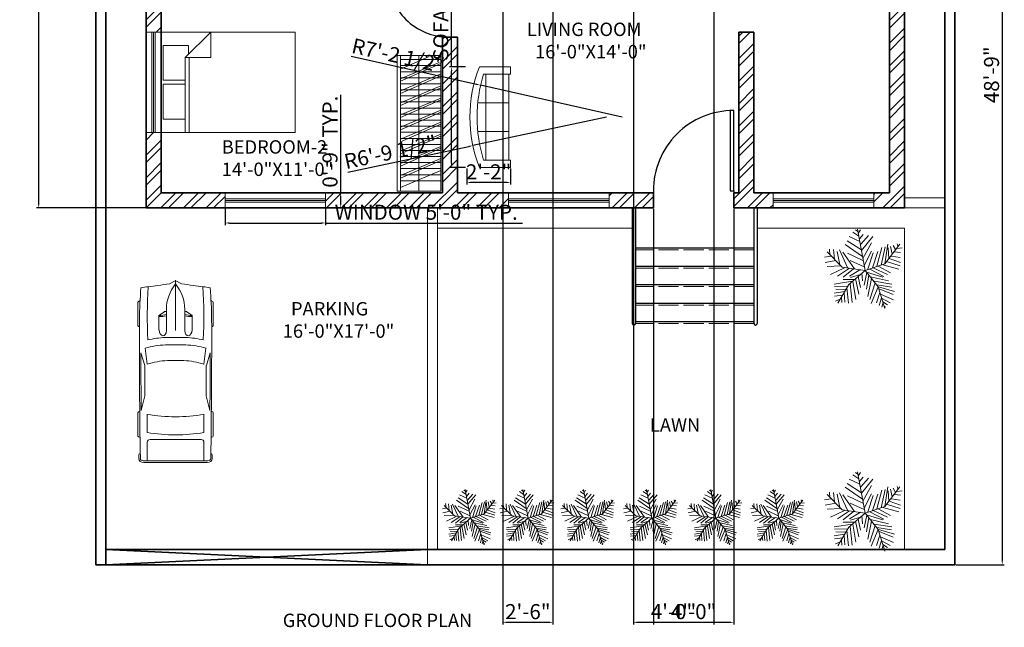
# Model space of a CAD drawing. Units: inches. Extents: x 451 to 1761, y 2292 to 3014.
# Tile 1 of 3: x 451 to 1039, y 2292 to 2655. Entities that reach past the tile are written whole.
import ezdxf

# ---------------------------------------------------------------- set-up
doc = ezdxf.new("R2010")
doc.units = ezdxf.units.IN
doc.linetypes.add('ACAD_ISO02W100', pattern=[15, 12, -3])
for name, color, linetype, lineweight in [('A-ANNO-DIMS', 2, 'Continuous', 18), ('A-ANNO-TEXT', 7, 'Continuous', 25), ('A-AREA-IDEN', 7, 'Continuous', 18), ('A-DOOR', 4, 'Continuous', 25), ('A-FLOR-CASE', 9, 'Continuous', 18), ('A-FLOR-CASE-PATT', 252, 'Continuous', 13), ('A-FLOR-STRS', 7, 'Continuous', 25), ('A-FLOR-STRS-HIDN', 8, 'ACAD_ISO02W100', 13), ('A-FURN', 8, 'Continuous', 18), ('A-GLAZ', 244, 'Continuous', 18), ('A-WALL', 7, 'Continuous', 35), ('A-WALL-PATT', 252, 'Continuous', 13), ('C-PROP', 7, 'Continuous', 35), ('C-SITE', 8, 'Continuous', 18), ('C-SITE-VEHC', 9, 'Continuous', 18), ('L-PLNT', 3, 'Continuous', 18)]:
    doc.layers.add(name, color=color, linetype=linetype, lineweight=lineweight)
doc.styles.get("Standard").update_dxf_attribs({"font": 'arial.ttf'})
doc.dimstyles.new('ISO-25', dxfattribs={"dimtxt": 9, "dimasz": 2.5, "dimexe": 1.25, "dimexo": 0.625, "dimtad": 1, "dimlunit": 3, "dimtxsty": 'Standard', "dimcen": 2.5, "dimadec": 0, "dimazin": 0, "dimtfac": 1, "dimtmove": 0, "dimatfit": 3, "dimfxl": 1, "dimarcsym": 0})

# ---------------------------------------------------------------- blocks, each defined once
blk = doc.blocks.new('*U3')
for p, q in [((0, 0), (0, 6)), ((40, 0), (40, 6))]:
    blk.add_line(p, q)
blk.add_lwpolyline([(0, 0), (0, -40), (1.75, -40), (1.75, 0)], close=True)
blk.add_arc((0, 0), 40, 270, 0)
blk = doc.blocks.new('Bed - Queen')
for p, q in [((0, -80.00003), (0, 0)), ((0, 0), (59.99999, 0)), ((59.99999, 0), (59.99999, -80.00003)), ((7.99999, -1.2), (28.79998, -1.2)), ((7.99999, -14.4), (7.99999, -1.2)), ((28.79998, -1.2), (28.79998, -14.4)), ((31.19999, -1.2), (51.99999, -1.2)), ((31.19999, -14.4), (31.19999, -1.2)), ((51.99999, -1.2), (51.99999, -16.4)), ((0, -14.4), (44.8, -14.4)), ((44.8, -16.8), (0, -16.8)), ((59.99999, -29.6), (44.8, -14.4)), ((44.8, -14.4), (44.8, -29.6)), ((51.99999, -16.4), (46.79936, -16.4)), ((44.8, -29.6), (59.99999, -29.6)), ((59.99999, -80.00003), (0, -80.00003))]:
    blk.add_line(p, q)
blk = doc.blocks.new('Sofa - Roundback 7 ft.')
for p, q in [((-12.00002, -32.4421), (-12.00003, -6.5971)), ((11.99997, -32.4421), (11.99998, -6.5971)), ((-36.000027, -34), (-36.000027, -11.4696)), ((-35.999844, -13.3819), (35.9998, -13.3819)), ((35.99998, -34), (35.99998, -11.4696)), ((-36.000027, -32.4421), (35.99998, -32.4421))]:
    blk.add_line(p, q)
for points in [[(-36.000027, -34), (-42.000027, -34), (-42.000027, -8)], [(41.99998, -8), (41.99998, -34), (35.99998, -34)]]:
    blk.add_lwpolyline(points)
for centre, radius, start, end in [((0, -114.25), 114.25, 68.43141, 111.5686), ((-0.00001, -127.1968), 121.1968, 72.72033, 107.2797)]:
    blk.add_arc(centre, radius, start, end)
blk = doc.blocks.new('*U12')
for p, q in [((-10.186, 53.64), (-13.084, 55.962)), ((0, 0), (-10.5, 57)), ((-9.099, 51.782), (-6.563, 55.962)), ((-7.288, 39.707), (-21.778, 46.673)), ((-8.737, 47.138), (-17.069, 52.711)), ((-7.65, 43.423), (-2.578, 49.46)), ((-5.839, 35.992), (4.667, 48.067)), ((-5.114, 27.632), (10.463, 46.673)), ((-48.585, 21.131), (-49.309, 29.026)), ((-43.513, 28.561), (-42.427, 15.558)), ((-35.544, 28.097), (-24.314, 3.947)), ((-3.665, 19.273), (-27.574, 35.527)), ((-5.114, 28.097), (-24.676, 40.636)), ((-2.941, 16.486), (8.652, 37.85)), ((16.259, 5.805), (23.142, 31.348)), ((22.055, 7.198), (27.489, 32.277)), ((27, 9), (48, 36)), ((27.127, 9.056), (31.112, 35.992)), ((31.836, 30.883), (32.561, 16.486)), ((35.096, 32.741), (37.27, 22.524)), ((38.719, 34.134), (41.979, 28.561)), ((43.791, 29.954), (51.036, 30.883)), ((44.153, 36.456), (45.239, 32.741)), ((-47.498, 19.737), (-55.83, 18.344)), ((-40.615, 13.7), (-55.105, 10.913)), ((-31.5, 4.5), (-52.5, 25.5)), ((-38.442, 26.239), (-34.819, 7.663)), ((-14.533, 2.09), (-30.834, 25.31)), ((-24.314, 23.917), (-2.941, 13.7)), ((-20.691, 13.7), (-1.129, 4.876)), ((-1.129, 6.734), (9.014, 26.704)), ((3.942, 1.625), (11.187, 24.381)), ((10.101, 3.483), (17.708, 26.239)), ((33.285, 16.486), (48.862, 10.913)), ((36.183, 19.737), (48.137, 17.88)), ((40.53, 25.775), (48.862, 24.846)), ((-33.37, 6.269), (-52.207, 5.34)), ((-28.299, 3.483), (-47.86, -5.805)), ((-21.416, 3.018), (-38.079, -8.128)), ((0, 0), (-31.5, 4.5)), ((-15.982, 2.09), (-30.11, -9.521)), ((0, 0), (-22.5, -19.5)), ((-6.563, 1.161), (-21.416, -8.128)), ((0, 0), (27, 9)), ((0, 0), (18, -22.5)), ((6.478, 1.625), (26.04, -8.592)), ((11.187, 3.483), (30.749, -5.805)), ((18.07, 5.805), (35.096, -3.483)), ((24.229, 7.663), (46.688, 1.625)), ((29.662, 12.307), (48.137, 6.269)), ((-15.257, -12.772), (-30.11, -12.772)), ((-6.563, -5.805), (-19.967, -9.985)), ((-13.446, -11.378), (-8.737, -32.741)), ((-9.461, -8.592), (-6.201, -23.453)), ((-4.752, -3.483), (-3.665, -14.629)), ((2.493, -3.019), (-1.491, -20.202)), ((1.769, -2.555), (24.229, -9.521)), ((5.029, -6.27), (2.131, -25.775)), ((9.014, -11.378), (3.58, -35.992)), ((7.565, -9.056), (32.198, -14.629)), ((-17.431, -15.094), (-42.789, -18.809)), ((-24.314, -21.596), (-42.427, -22.06)), ((-26.849, -26.24), (-40.253, -25.775)), ((-22.5, -19.5), (-37.5, -45)), ((-25.038, -23.918), (-22.865, -45.281)), ((-20.691, -18.345), (-17.793, -44.352)), ((-17.069, -15.094), (-12.721, -40.172)), ((14.085, -16.951), (6.478, -40.172)), ((18.07, -22.524), (8.289, -45.745)), ((12.274, -15.094), (36.907, -18.809)), ((16.259, -19.738), (36.183, -22.989)), ((18, -22.5), (27, -52.5)), ((18.433, -22.524), (40.53, -29.026)), ((19.157, -25.311), (38.719, -33.206)), ((-28.299, -29.026), (-42.789, -31.348)), ((-30.834, -34.135), (-42.427, -35.528)), ((-34.457, -39.708), (-40.978, -42.494)), ((-32.646, -36.921), (-31.921, -44.352)), ((-29.023, -30.884), (-27.936, -43.887)), ((20.244, -30.419), (15.897, -44.816)), ((22.78, -37.85), (19.519, -48.532)), ((21.331, -32.741), (39.081, -40.636)), ((22.78, -38.314), (34.372, -44.816)), ((24.591, -45.745), (23.142, -50.854)), ((24.591, -43.423), (30.749, -47.603)), ((26.764, -49.925), (28.213, -50.854))]:
    blk.add_line(p, q)
blk = doc.blocks.new('*D13')
at = {"layer": 'A-ANNO-DIMS', "color": 0, "lineweight": -2, "transparency": 16777216}
for p, q in [((1010.42, 2914.76), (1039.33, 2914.76)), ((1038.08, 2912.26), (1038.08, 2332.26)), ((1010.42, 2329.76), (1039.33, 2329.76))]:
    blk.add_line(p, q, dxfattribs=at)
at = {"layer": 'A-ANNO-DIMS', "color": 0, "transparency": 16777216}
for points in [[(1037.66, 2912.26), (1038.49, 2912.26), (1038.08, 2914.76)], [(1037.66, 2332.26), (1038.49, 2332.26), (1038.08, 2329.76)]]:
    blk.add_solid(points, dxfattribs=at)
at = {"layer": 'Defpoints', "color": 0, "transparency": 16777216}
for p in [(1009.79, 2914.76), (1009.79, 2329.76), (1038.08, 2329.76)]:
    blk.add_point(p, dxfattribs=at)
at = {"layer": 'A-ANNO-DIMS', "color": 0, "transparency": 16777216, "insert": (1032.86, 2622.26), "char_height": 9, "attachment_point": 5, "rotation": 90}
blk.add_mtext('48\'-9"', dxfattribs=at)
blk = doc.blocks.new('*U18')
for p, q in [((21.1, 37.4), (21.1, 36.8)), ((46.6, 38.9), (22.4, 38.9)), ((47.8, 37.4), (47.8, 37.4)), ((70, 31.5), (86.4, 29.4)), ((88, 31.9), (74.8, 35.9)), ((134.3, 35.6), (119.3, 31.8)), ((135.5, 37.1), (135.5, 37.4)), ((136.7, 38.9), (160.9, 38.9)), ((162.1, 37.4), (162.1, 36.8)), ((186.5, -33.5), (186.5, 33.5)), ((188.4, -32.8), (188.4, 32.8)), ((138.4, 29.4), (157.2, 29.4)), ((164.5, 26.4), (164.5, -26.4)), ((186.5, 29.4), (167, 29.4)), ((32.1, 9.5), (32.1, 11.2)), ((32.3, 11.6), (36.1, 17.2)), ((36.1, 17.2), (50.9, 17.2)), ((58.9, -10.8), (58.9, 10.8)), ((66.6, -10.5), (66.6, 10.5)), ((186.5, -10.5), (186.5, 10.5)), ((3.3, 6.1), (0.1, 0.4)), ((29.8, 9.5), (51.7, 9.5)), ((82.7, 8.5), (82.7, -8.5)), ((0, 0), (51.7, 0)), ((0.1, -0.4), (3.3, -6.1)), ((29.8, -9.5), (51.7, -9.5)), ((32.1, -9.5), (32.1, -11.2)), ((32.3, -11.6), (36.1, -17.2)), ((36.1, -17.2), (50.9, -17.2)), ((86.4, -29.4), (70, -31.5)), ((157.2, -29.4), (138.4, -29.4)), ((167, -29.4), (186.5, -29.4)), ((21.1, -37.4), (21.1, -36.8)), ((46.6, -38.9), (22.4, -38.9)), ((47.8, -37.4), (47.8, -37.4)), ((88, -31.9), (74.8, -35.9)), ((134.3, -35.6), (119.3, -31.8)), ((135.5, -37.1), (135.5, -37.4)), ((136.7, -38.9), (160.9, -38.9)), ((162.1, -37.4), (162.1, -36.8))]:
    blk.add_line(p, q)
for centre, major_axis, ratio, start_param, end_param in [((266, -27.5), (0, 313.3), 0.842304, 1.367076, 1.39176), ((41.2, -490.9), (0, 528.2), 0.842304, 0.00281, 0.075598), ((22.4, 37.4), (0, -1.48), 0.842304, 3.141593, 4.712389), ((64.5, -10555.6), (0, 10593), 0.842304, -0.013397, 0.002797), ((46.6, 37.4), (0, 1.48), 0.842304, -1.570796, 0), ((135.3, 5.4), (0, 81.8), 0.842304, 1.245306, 1.50788), ((64.5, -10555.6), (0, -10591.5), 0.842304, 3.133765, 3.140441), ((95.8, -3666.4), (0, -3698.2), 0.842304, 3.134049, 3.144098), ((136.7, 37.4), (0, -1.48), 0.842304, 3.141593, 4.712389), ((160.9, 37.4), (0, 1.48), 0.842304, -1.570796, 0), ((180.6, 35.8), (0, 2.22), 0.842304, -0.013017, 1.249894), ((64.5, -10556.4), (0, 10595.3), 0.842304, -0.013397, -0.013017), ((184, 32.8), (0, -5.25), 0.842304, 1.570796, 3.128196), ((184, 33.5), (0, -2.96), 0.842304, 1.570796, 3.128196), ((259.2, -27.5), (0, -305.3), 0.842304, 4.528606, 4.561838), ((37.5, -594), (0, -623.3), 0.842304, 3.096046, 3.200911), ((134.4, 5.4), (0, -89.8), 0.842304, 4.449482, 4.652344), ((149.6, 2.8), (0, -79.6), 0.842304, 4.372215, 4.640744), ((17.1, 0), (0, 147), 0.842304, 4.511394, 4.913384), ((35.9, 0), (0, 147), 0.842304, 4.511394, 4.913384), ((167, 26.4), (0, 2.96), 0.842304, 0, 1.570796), ((-204.5, 52.4), (0, -251), 0.842304, 1.385369, 1.434372), ((32.7, 11.2), (0, 0.74), 0.842304, 0.879714, 1.570796), ((13, 17), (0, 27.4), 0.842304, 4.435146, 4.718221), ((14.2, 17), (0, 27.4), 0.842304, 4.435146, 4.718221), ((50.8, 13.3), (6.34, -0.36), 0.603834, -1.395552, 1.581315), ((0.6, 0), (0, -0.74), 0.842304, 4.131459, 5.293319), ((29.8, -46.7), (0, 56.2), 0.842304, 0, 0.590319), ((-204.5, -52.4), (0, 251), 0.842304, -1.434372, -1.385369), ((29.8, 46.7), (0, 56.2), 0.842304, 2.551274, 3.141593), ((13, -17), (0, -27.4), 0.842304, 1.564964, 1.848039), ((14.2, -17), (0, -27.4), 0.842304, 1.564964, 1.848039), ((149.6, -2.8), (0, -79.6), 0.842304, -1.499151, -1.230623), ((259.2, 27.5), (0, 305.3), 0.842304, 1.721348, 1.754579), ((32.7, -11.2), (0, -0.74), 0.842304, 4.712389, 5.403472), ((134.4, -5.4), (0, -89.8), 0.842304, -1.510751, -1.307889), ((135.3, -5.4), (0, -81.8), 0.842304, -1.50788, -1.245306), ((266, 27.5), (0, 313.3), 0.842304, 1.749832, 1.774517), ((37.5, 594), (0, -623.3), 0.842304, -0.059319, 0.045547), ((167, -26.4), (0, -2.96), 0.842304, 4.712389, 6.283185), ((41.2, 490.9), (0, -528.2), 0.842304, -0.075598, -0.00281), ((22.4, -37.4), (0, 1.48), 0.842304, 1.570796, 3.141593), ((64.5, 10555.6), (0, 10593), 0.842304, 3.138796, 3.15499), ((46.6, -37.4), (0, -1.48), 0.842304, 0, 1.570796), ((64.5, 10555.6), (0, -10591.5), 0.842304, 0.001152, 0.007828), ((95.8, 3666.4), (0, -3698.2), 0.842304, -0.002505, 0.007544), ((136.7, -37.4), (0, -1.48), 0.842304, -1.570796, 0), ((160.9, -37.4), (0, 1.48), 0.842304, 3.141593, 4.712389), ((180.6, -35.8), (0, -2.22), 0.842304, -1.249894, 0.013017), ((64.5, 10556.4), (0, 10595.3), 0.842304, 3.15461, 3.15499), ((184, -32.8), (0, -5.25), 0.842304, 0.013397, 1.570796), ((184, -33.5), (0, 2.96), 0.842304, 3.15499, 4.712389)]:
    blk.add_ellipse(centre, major_axis=major_axis, ratio=ratio, start_param=start_param, end_param=end_param)
at = {"extrusion": (0, 0, -1)}
blk.add_ellipse((50.8, -13.3), major_axis=(6.34, 0.36), ratio=0.603834, start_param=-1.395552, end_param=1.581315, dxfattribs=at)
blk = doc.blocks.new('WIN-60IN')
for p, q in [((0, 5.5), (60, 5.5)), ((0, 4.5), (60, 4.5)), ((0, 3.5), (60, 3.5))]:
    blk.add_line(p, q)
blk.add_lwpolyline([(0, 0), (0, 9), (60, 9), (60, 0)], close=True)
blk = doc.blocks.new('*D24')
at = {"layer": 'A-ANNO-DIMS', "color": 0, "lineweight": -2, "transparency": 16777216}
for p, q in [((574.03, 2542.13), (574.03, 2532.51)), ((634.03, 2542.13), (634.03, 2532.51)), ((576.53, 2533.76), (631.53, 2533.76)), ((634.03, 2533.76), (751.66, 2533.76))]:
    blk.add_line(p, q, dxfattribs=at)
at = {"layer": 'A-ANNO-DIMS', "color": 0, "transparency": 16777216}
for points in [[(576.53, 2534.18), (576.53, 2533.34), (574.03, 2533.76)], [(631.53, 2534.18), (631.53, 2533.34), (634.03, 2533.76)]]:
    blk.add_solid(points, dxfattribs=at)
at = {"layer": 'Defpoints', "color": 0, "transparency": 16777216}
for p in [(574.03, 2542.76), (634.03, 2542.76), (634.03, 2533.76)]:
    blk.add_point(p, dxfattribs=at)
at = {"layer": 'A-ANNO-DIMS', "color": 0, "transparency": 16777216, "insert": (694.1, 2539.04), "char_height": 9, "attachment_point": 5}
blk.add_mtext('WINDOW 5\'-0" TYP.', dxfattribs=at)
blk = doc.blocks.new('*D25')
at = {"layer": 'A-ANNO-DIMS', "color": 0, "lineweight": -2, "transparency": 16777216}
for p, q in [((643.03, 2551.76), (643.03, 2610.37)), ((634.65, 2551.76), (644.28, 2551.76)), ((643.03, 2545.26), (643.03, 2549.26)), ((634.65, 2542.76), (644.28, 2542.76))]:
    blk.add_line(p, q, dxfattribs=at)
at = {"layer": 'A-ANNO-DIMS', "color": 0, "transparency": 16777216}
for points in [[(642.61, 2549.26), (643.44, 2549.26), (643.03, 2551.76)], [(642.61, 2545.26), (643.44, 2545.26), (643.03, 2542.76)]]:
    blk.add_solid(points, dxfattribs=at)
at = {"layer": 'Defpoints', "color": 0, "transparency": 16777216}
for p in [(634.03, 2551.76), (643.03, 2551.76), (634.03, 2542.76)]:
    blk.add_point(p, dxfattribs=at)
at = {"layer": 'A-ANNO-DIMS', "color": 0, "transparency": 16777216, "insert": (637.81, 2582.31), "char_height": 9, "attachment_point": 5, "rotation": 90}
blk.add_mtext('0\'-9" TYP.', dxfattribs=at)
blk = doc.blocks.new('*D32')
at = {"layer": 'A-ANNO-DIMS', "color": 0, "lineweight": -2, "transparency": 16777216}
for p, q in [((709.28, 2626.98), (709.28, 2692.34)), ((717.66, 2626.98), (708.03, 2626.98)), ((709.28, 2569.48), (709.28, 2624.48)), ((717.66, 2566.98), (708.03, 2566.98))]:
    blk.add_line(p, q, dxfattribs=at)
at = {"layer": 'A-ANNO-DIMS', "color": 0, "transparency": 16777216}
for points in [[(708.87, 2624.48), (709.7, 2624.48), (709.28, 2626.98)], [(708.87, 2569.48), (709.7, 2569.48), (709.28, 2566.98)]]:
    blk.add_solid(points, dxfattribs=at)
at = {"layer": 'Defpoints', "color": 0, "transparency": 16777216}
for p in [(709.28, 2626.98), (718.28, 2626.98), (718.28, 2566.98)]:
    blk.add_point(p, dxfattribs=at)
at = {"layer": 'A-ANNO-DIMS', "color": 0, "transparency": 16777216, "insert": (704, 2660.91), "char_height": 9, "attachment_point": 5, "rotation": 90}
blk.add_mtext('SOFA 5\'-0"', dxfattribs=at)
blk = doc.blocks.new('*D33')
at = {"layer": 'A-ANNO-DIMS', "color": 0, "lineweight": -2, "transparency": 16777216}
for p, q in [((718.28, 2566.36), (718.28, 2556.73)), ((744.47, 2566.36), (744.47, 2556.73)), ((741.97, 2557.98), (720.78, 2557.98))]:
    blk.add_line(p, q, dxfattribs=at)
at = {"layer": 'A-ANNO-DIMS', "color": 0, "transparency": 16777216}
for points in [[(720.78, 2558.4), (720.78, 2557.57), (718.28, 2557.98)], [(741.97, 2558.4), (741.97, 2557.57), (744.47, 2557.98)]]:
    blk.add_solid(points, dxfattribs=at)
at = {"layer": 'Defpoints', "color": 0, "transparency": 16777216}
for p in [(718.28, 2566.98), (744.47, 2566.98), (718.28, 2557.98)]:
    blk.add_point(p, dxfattribs=at)
at = {"layer": 'A-ANNO-DIMS', "color": 0, "transparency": 16777216, "insert": (731.38, 2563.13), "char_height": 9, "attachment_point": 5}
blk.add_mtext('2\'-2"', dxfattribs=at)
blk = doc.blocks.new('*D35')
at = {"layer": 'A-ANNO-DIMS', "color": 0, "lineweight": -2, "transparency": 16777216}
for p, q in [((526.17, 2914.76), (461.44, 2914.76)), ((462.69, 2545.26), (462.69, 2912.26)), ((526.17, 2542.76), (461.44, 2542.76))]:
    blk.add_line(p, q, dxfattribs=at)
at = {"layer": 'A-ANNO-DIMS', "color": 0, "transparency": 16777216}
for points in [[(462.27, 2912.26), (463.11, 2912.26), (462.69, 2914.76)], [(462.27, 2545.26), (463.11, 2545.26), (462.69, 2542.76)]]:
    blk.add_solid(points, dxfattribs=at)
at = {"layer": 'Defpoints', "color": 0, "transparency": 16777216}
for p in [(462.69, 2914.76), (526.79, 2914.76), (526.79, 2542.76)]:
    blk.add_point(p, dxfattribs=at)
at = {"layer": 'A-ANNO-DIMS', "color": 0, "transparency": 16777216, "insert": (457.47, 2728.76), "char_height": 9, "attachment_point": 5, "rotation": 90}
blk.add_mtext('31\'-0"', dxfattribs=at)
blk = doc.blocks.new('*D37')
at = {"layer": 'A-ANNO-DIMS', "color": 0, "lineweight": -2, "transparency": 16777216}
for p, q in [((829.79, 2542.13), (829.79, 2294.1)), ((877.79, 2542.13), (877.79, 2294.1)), ((832.29, 2295.35), (875.29, 2295.35))]:
    blk.add_line(p, q, dxfattribs=at)
at = {"layer": 'A-ANNO-DIMS', "color": 0, "transparency": 16777216}
for points in [[(832.29, 2295.77), (832.29, 2294.93), (829.79, 2295.35)], [(875.29, 2295.77), (875.29, 2294.93), (877.79, 2295.35)]]:
    blk.add_solid(points, dxfattribs=at)
at = {"layer": 'Defpoints', "color": 0, "transparency": 16777216}
for p in [(829.79, 2542.76), (877.79, 2542.76), (877.79, 2295.35)]:
    blk.add_point(p, dxfattribs=at)
at = {"layer": 'A-ANNO-DIMS', "color": 0, "transparency": 16777216, "insert": (853.79, 2300.57), "char_height": 9, "attachment_point": 5}
blk.add_mtext('4\'-0"', dxfattribs=at)
blk = doc.blocks.new('*D38')
at = {"layer": 'A-ANNO-DIMS', "color": 0, "lineweight": -2, "transparency": 16777216}
for p, q in [((817.79, 2776.13), (817.79, 2294.1)), ((865.79, 2776.13), (865.79, 2294.1)), ((820.29, 2295.35), (863.29, 2295.35))]:
    blk.add_line(p, q, dxfattribs=at)
at = {"layer": 'A-ANNO-DIMS', "color": 0, "transparency": 16777216}
for points in [[(820.29, 2295.77), (820.29, 2294.93), (817.79, 2295.35)], [(863.29, 2295.77), (863.29, 2294.93), (865.79, 2295.35)]]:
    blk.add_solid(points, dxfattribs=at)
at = {"layer": 'Defpoints', "color": 0, "transparency": 16777216}
for p in [(817.79, 2776.76), (865.79, 2776.76), (865.79, 2295.35)]:
    blk.add_point(p, dxfattribs=at)
at = {"layer": 'A-ANNO-DIMS', "color": 0, "transparency": 16777216, "insert": (841.79, 2300.57), "char_height": 9, "attachment_point": 5}
blk.add_mtext('4\'-0"', dxfattribs=at)
blk = doc.blocks.new('*D39')
at = {"layer": 'A-ANNO-DIMS', "color": 0, "lineweight": -2, "transparency": 16777216}
for p, q in [((739.79, 2812.13), (739.79, 2294.1)), ((769.79, 2812.13), (769.79, 2294.1)), ((742.29, 2295.35), (767.29, 2295.35))]:
    blk.add_line(p, q, dxfattribs=at)
at = {"layer": 'A-ANNO-DIMS', "color": 0, "transparency": 16777216}
for points in [[(742.29, 2295.77), (742.29, 2294.93), (739.79, 2295.35)], [(767.29, 2295.77), (767.29, 2294.93), (769.79, 2295.35)]]:
    blk.add_solid(points, dxfattribs=at)
at = {"layer": 'Defpoints', "color": 0, "transparency": 16777216}
for p in [(739.79, 2812.76), (769.79, 2812.76), (769.79, 2295.35)]:
    blk.add_point(p, dxfattribs=at)
at = {"layer": 'A-ANNO-DIMS', "color": 0, "transparency": 16777216, "insert": (754.79, 2300.57), "char_height": 9, "attachment_point": 5}
blk.add_mtext('2\'-6"', dxfattribs=at)
blk = doc.blocks.new('*D48')
at = {"layer": 'A-ANNO-DIMS', "color": 0, "lineweight": -2, "transparency": 16777216}
for p, q in [((649.21, 2633.44), (724.15, 2616.56)), ((811.04, 2596.98), (726.59, 2616.01))]:
    blk.add_line(p, q, dxfattribs=at)
at = {"layer": 'A-ANNO-DIMS', "color": 0, "transparency": 16777216}
blk.add_solid([(724.24, 2616.96), (724.06, 2616.15), (726.59, 2616.01)], dxfattribs=at)
at = {"layer": 'Defpoints', "color": 0, "transparency": 16777216}
for p in [(726.59, 2616.01), (811.04, 2596.98)]:
    blk.add_point(p, dxfattribs=at)
at = {"layer": 'A-ANNO-DIMS', "color": 0, "transparency": 16777216, "insert": (677.08, 2632.57), "char_height": 9, "attachment_point": 5, "rotation": 347.30544}
blk.add_mtext('R7\'-2 1/2"', dxfattribs=at)
blk = doc.blocks.new('*D49')
at = {"layer": 'A-ANNO-DIMS', "color": 0, "lineweight": -2, "transparency": 16777216}
for p, q in [((801.8, 2596.98), (721.98, 2580)), ((647.3, 2564.11), (719.53, 2579.48))]:
    blk.add_line(p, q, dxfattribs=at)
at = {"layer": 'A-ANNO-DIMS', "color": 0, "transparency": 16777216}
blk.add_solid([(719.44, 2579.89), (719.62, 2579.07), (721.98, 2580)], dxfattribs=at)
at = {"layer": 'Defpoints', "color": 0, "transparency": 16777216}
for p in [(801.8, 2596.98), (721.98, 2580)]:
    blk.add_point(p, dxfattribs=at)
at = {"layer": 'A-ANNO-DIMS', "color": 0, "transparency": 16777216, "insert": (672.98, 2574.97), "char_height": 9, "attachment_point": 5, "rotation": 12.01201}
blk.add_mtext('R6\'-9 1/2"', dxfattribs=at)

msp = doc.modelspace()

# ---------------------------------------------------------------- hatches: boundary and pattern name
at = {"layer": 'A-FLOR-CASE-PATT'}
h = msp.add_hatch(dxfattribs=at)
h.set_pattern_fill('ANSI31', color=256, scale=2.09659, angle=-22.1278, style=0)
h.paths.add_polyline_path([(678.791, 2552.759), (702.791, 2562.883), (702.791, 2627.905), (699.385, 2633.693), (678.791, 2625.006)])
h = msp.add_hatch(dxfattribs=at)
h.set_pattern_fill('ANSI31', color=256, scale=2.08217, angle=-21.2114, style=0)
h.paths.add_polyline_path([(678.791, 2556.222), (702.791, 2566.801), (702.791, 2631.824), (690.643, 2633.693), (678.791, 2628.469)])
h = msp.add_hatch(dxfattribs=at)
h.set_pattern_fill('ANSI31', color=256, scale=1.13999, angle=-45, style=0)
h.paths.add_polyline_path([(678.791, 2556.222), (702.791, 2556.222), (702.791, 2632.23), (678.791, 2632.23)])
at = {"layer": 'A-WALL-PATT'}
h = msp.add_hatch(dxfattribs=at)
h.set_pattern_fill('ANSI32', color=256)
h.paths.add_polyline_path([(703.791, 2551.759), (634.026, 2551.759), (634.026, 2542.759), (743.266, 2542.759), (743.266, 2551.759), (712.791, 2551.759), (712.791, 2644.759), (707.391, 2644.759), (703.791, 2644.759)])
h.paths.add_polyline_path([(535.791, 2551.759), (535.791, 2587.758), (526.791, 2587.758), (526.791, 2542.759), (574.026, 2542.759), (574.026, 2551.759)])
h.paths.add_polyline_path([(526.791, 2647.758), (535.791, 2647.758), (535.791, 2683.759), (619.791, 2683.759), (619.791, 2692.759), (535.791, 2692.759), (535.791, 2726.772), (526.791, 2726.772)])
h.paths.add_polyline_path([(649.791, 2692.759), (649.791, 2683.759), (703.791, 2683.759), (703.791, 2680.759), (712.791, 2680.759), (712.791, 2752.759), (712.791, 2764.759), (703.791, 2764.759), (703.791, 2761.759), (535.791, 2761.759), (535.791, 2804.959), (526.791, 2804.959), (526.791, 2747.772), (535.791, 2747.772), (535.791, 2752.759), (703.791, 2752.759), (703.791, 2692.759)])
h.paths.add_polyline_path([(781.791, 2785.759), (781.791, 2905.759), (811.791, 2905.759), (811.791, 2914.759), (763.791, 2914.759), (763.791, 2905.759), (772.791, 2905.759), (772.791, 2821.759), (769.791, 2821.759), (769.791, 2812.759), (772.791, 2812.759), (772.791, 2776.759), (817.791, 2776.759), (817.791, 2785.759)])
h.paths.add_polyline_path([(703.791, 2800.759), (712.791, 2800.759), (712.791, 2812.759), (739.791, 2812.759), (739.791, 2821.759), (712.791, 2821.759), (712.791, 2905.759), (742.791, 2905.759), (742.791, 2914.759), (649.791, 2914.759), (649.791, 2905.759), (703.791, 2905.759)])
h.paths.add_polyline_path([(526.791, 2864.959), (535.791, 2864.959), (535.791, 2905.759), (589.791, 2905.759), (589.791, 2914.759), (526.791, 2914.759)])
h.paths.add_polyline_path([(901.791, 2905.759), (901.791, 2875.759), (910.791, 2875.759), (910.791, 2905.759), (916.791, 2905.759), (916.791, 2914.759), (871.791, 2914.759), (871.791, 2905.759)])
h.paths.add_polyline_path([(901.791, 2785.759), (865.791, 2785.759), (865.791, 2776.759), (901.791, 2776.759), (913.791, 2776.759), (913.791, 2781.259), (913.791, 2785.759), (910.791, 2785.759), (910.791, 2815.759), (901.791, 2815.759)])
h.paths.add_polyline_path([(979.791, 2914.759), (964.791, 2914.759), (964.791, 2905.759), (970.791, 2905.759), (970.791, 2785.759), (943.791, 2785.759), (943.791, 2776.759), (970.791, 2776.759), (970.791, 2551.759), (961.316, 2551.759), (961.316, 2542.759), (979.791, 2542.759)])
h.paths.add_polyline_path([(901.316, 2542.759), (901.316, 2551.759), (889.791, 2551.759), (889.791, 2647.758), (880.791, 2647.758), (880.791, 2551.759), (877.791, 2551.759), (877.791, 2542.759)])
h.paths.add_polyline_path([(803.266, 2551.759), (803.266, 2542.759), (829.791, 2542.759), (829.791, 2551.759)])

# ---------------------------------------------------------------- linework, layer by layer
at = {"layer": 'A-FLOR-CASE'}
for p, q in [((676.791, 2633.693), (676.791, 2552.759)), ((676.791, 2633.693), (702.791, 2633.693)), ((678.791, 2633.693), (678.791, 2552.759)), ((689.791, 2633.693), (689.791, 2552.759)), ((702.791, 2633.693), (702.791, 2552.759)), ((676.791, 2552.759), (702.791, 2552.759))]:
    msp.add_line(p, q, dxfattribs=at)
at = {"layer": 'A-FLOR-STRS'}
for p, q in [((817.178, 2542.759), (817.178, 2473.759)), ((819.178, 2542.759), (819.178, 2473.759)), ((889.791, 2542.759), (889.791, 2473.759)), ((891.791, 2542.759), (891.791, 2473.759)), ((889.791, 2518.759), (819.178, 2518.759)), ((889.791, 2507.759), (819.178, 2507.759)), ((889.791, 2496.759), (819.178, 2496.759)), ((889.791, 2485.759), (819.178, 2485.759)), ((889.791, 2474.759), (819.178, 2474.759))]:
    msp.add_line(p, q, dxfattribs=at)
for centre in [(818.178, 2473.815), (890.791, 2473.815)]:
    msp.add_arc(centre, 1.002, 183.206796, 356.793204, dxfattribs=at)
at = {"layer": 'A-FLOR-STRS-HIDN'}
for p, q in [((889.791, 2517.759), (819.178, 2517.759)), ((889.791, 2506.759), (819.178, 2506.759)), ((889.791, 2495.759), (819.178, 2495.759)), ((889.791, 2484.759), (819.178, 2484.759)), ((889.791, 2473.759), (819.178, 2473.759))]:
    msp.add_line(p, q, dxfattribs=at)
at = {"layer": 'A-WALL'}
for p, q in [((526.791, 2914.759), (526.791, 2542.759)), ((979.791, 2914.759), (979.791, 2542.759)), ((970.791, 2776.759), (970.791, 2551.759)), ((535.791, 2683.759), (535.791, 2551.759)), ((880.791, 2647.758), (880.791, 2551.759)), ((889.791, 2647.758), (880.791, 2647.758)), ((889.791, 2647.758), (889.791, 2551.759)), ((703.791, 2644.759), (712.791, 2644.759)), ((703.791, 2644.759), (703.791, 2551.759)), ((712.791, 2644.759), (712.791, 2551.759)), ((535.791, 2551.759), (703.791, 2551.759)), ((712.791, 2551.759), (829.791, 2551.759)), ((829.791, 2551.759), (829.791, 2542.759)), ((877.791, 2551.759), (877.791, 2542.759)), ((877.791, 2551.759), (880.791, 2551.759)), ((889.791, 2551.759), (970.791, 2551.759)), ((526.791, 2542.759), (829.791, 2542.759)), ((877.791, 2542.759), (979.791, 2542.759))]:
    msp.add_line(p, q, dxfattribs=at)
at = {"layer": 'C-PROP'}
for p, q in [((496.791, 2914.759), (496.791, 2329.759)), ((1009.791, 2914.759), (1009.791, 2329.759)), ((502.791, 2905.759), (502.791, 2329.759)), ((1003.791, 2905.759), (1003.791, 2338.759)), ((502.791, 2338.759), (1003.791, 2338.759)), ((502.791, 2329.759), (694.791, 2338.759)), ((694.791, 2329.759), (502.791, 2338.759)), ((496.791, 2329.759), (1009.791, 2329.759))]:
    msp.add_line(p, q, dxfattribs=at)
at = {"layer": 'C-SITE'}
for p, q in [((979.791, 2551.336), (979.791, 2548.759)), ((979.791, 2548.759), (1003.791, 2548.759)), ((526.791, 2542.759), (502.791, 2542.759)), ((694.791, 2542.759), (694.791, 2329.759)), ((700.791, 2542.759), (700.791, 2338.759)), ((979.791, 2542.759), (1003.791, 2542.759)), ((700.791, 2530.759), (817.178, 2530.759)), ((891.791, 2530.759), (979.791, 2530.759)), ((979.791, 2530.759), (979.791, 2338.759))]:
    msp.add_line(p, q, dxfattribs=at)

# ---------------------------------------------------------------- block references
at = {"layer": 'A-DOOR'}
for p, xscale, yscale, zscale, rotation in [((707.391, 2680.759), 0.9000000000000111, 0.9000000000000111, 0.9000000000000111, 270), ((877.791, 2552.959), 1.199999999999999, 1.199999999999999, 1.199999999999999, 180)]:
    msp.add_blockref('*U3', p, dxfattribs=dict(at, xscale=xscale, yscale=yscale, zscale=zscale, rotation=rotation))
at = {"layer": 'A-FURN', "rotation": 90}
msp.add_blockref('Bed - Queen', (535.791, 2587.759), dxfattribs=at)
at = {"layer": 'A-FURN', "xscale": 0.7142856363870707, "yscale": 0.7142856363870707, "zscale": 0.7142856363870707, "rotation": 90}
msp.add_blockref('Sofa - Roundback 7 ft.', (720.188, 2596.983), dxfattribs=at)
at = {"layer": 'A-GLAZ', "rotation": 270}
msp.add_blockref('WIN-60IN', (526.792, 2647.758), dxfattribs=at)
at = {"layer": 'A-GLAZ'}
for p in [(574.026, 2542.759), (743.266, 2542.759), (901.316, 2542.759)]:
    msp.add_blockref('WIN-60IN', p, dxfattribs=at)
at = {"layer": 'C-SITE-VEHC', "xscale": 0.5769333709830182, "yscale": 0.5769333709830182, "zscale": 0.5769333709830182, "rotation": 270}
msp.add_blockref('*U18', (544.412, 2499.383), dxfattribs=at)
at = {"layer": 'L-PLNT'}
for p, xscale, yscale, zscale in [((956.205, 2505.478), 0.4329902194539378, 0.4329902194539378, 0.4329902194539378), ((956.205, 2360.577), 0.4329902194539378, 0.4329902194539378, 0.4329902194539378), ((720.556, 2357.488), 0.3010466794113964, 0.3010466794113964, 0.3010466794113964), ((754.913, 2357.488), 0.3010466794113964, 0.3010466794113964, 0.3010466794113964), ((791.273, 2357.488), 0.3010466794113964, 0.3010466794113964, 0.3010466794113964), ((828.787, 2357.488), 0.3010466794113964, 0.3010466794113964, 0.3010466794113964), ((867.135, 2357.488), 0.3010466794113964, 0.3010466794113964, 0.3010466794113964), ((904.649, 2357.488), 0.3010466794113964, 0.3010466794113964, 0.3010466794113964)]:
    msp.add_blockref('*U12', p, dxfattribs=dict(at, xscale=xscale, yscale=yscale, zscale=zscale))

# ---------------------------------------------------------------- texts
at = {"layer": 'A-ANNO-TEXT', "insert": (608.451, 2300.513), "char_height": 8, "attachment_point": 1}
msp.add_mtext_dynamic_manual_height_columns('GROUND FLOOR PLAN', width=134.00211, gutter_width=12.5, heights=[0], dxfattribs=at)
at = {"layer": 'A-AREA-IDEN', "char_height": 8, "attachment_point": 1}
for s, width, insert in [('LIVING ROOM \\P  16\'-0"X14\'-0"', 75.6515, (754.199, 2653.396)), ('BEDROOM-2 \\P14\'-0"X11\'-0"', 67.82233, (572.018, 2583.17)), ('  PARKING \\P16\'-0"X17\'-0"', 64.02122, (608.451, 2486.566)), ('LAWN', 32.42441, (827.713, 2417.119))]:
    msp.add_mtext_dynamic_manual_height_columns(s, width=width, gutter_width=12.5, heights=[0], dxfattribs=dict(at, insert=insert))

# ---------------------------------------------------------------- dimensions: what is measured, and where the dimension line sits
at = {"layer": 'A-ANNO-DIMS'}
for base, p1, p2, angle, override, picture, middle in [((462.691, 2914.759), (526.791, 2542.759), (526.791, 2914.759), 90, {"dimdec": 1, "dimlfac": 1, "dimrnd": 0, "dimzin": 1, "dimdsep": 46, "dimlunit": 4, "dimfrac": 2}, '*D35', (457.468, 2728.759)), ((1038.076, 2329.759), (1009.791, 2914.759), (1009.791, 2329.759), 90, {"dimclrd": 0, "dimclre": 0, "dimclrt": 0}, '*D13', (1032.856, 2622.259)), ((718.284, 2557.983), (744.474, 2566.983), (718.284, 2566.983), 180, {"dimdec": 1, "dimlfac": 1, "dimrnd": 0, "dimzin": 1, "dimdsep": 46, "dimlunit": 4, "dimfrac": 2}, '*D33', (731.379, 2563.126))]:
    dim = msp.add_linear_dim(base=base, p1=p1, p2=p2, angle=angle, dimstyle='ISO-25', override=override, dxfattribs=at)
    dim.commit()
    dim.dimension.update_dxf_attribs({"geometry": picture, "text_midpoint": middle})
for base, p1, p2, picture, middle in [((769.791, 2295.35), (739.791, 2812.759), (769.791, 2812.759), '*D39', (754.791, 2300.57)), ((865.791, 2295.35), (817.791, 2776.759), (865.791, 2776.759), '*D38', (841.791, 2300.57)), ((877.791, 2295.35), (829.791, 2542.759), (877.791, 2542.759), '*D37', (853.791, 2300.57))]:
    dim = msp.add_linear_dim(base=base, p1=p1, p2=p2, dimstyle='ISO-25', override={"dimdec": 1, "dimlfac": 1, "dimrnd": 0, "dimzin": 1, "dimdsep": 46, "dimlunit": 4, "dimfrac": 2}, dxfattribs=at)
    dim.commit()
    dim.dimension.update_dxf_attribs({"geometry": picture, "text_midpoint": middle})
for base, p1, p2, text, picture, middle in [((709.284, 2626.983), (718.284, 2566.983), (718.284, 2626.983), 'SOFA <>', '*D32', (704.002, 2660.911)), ((643.026, 2551.759), (634.026, 2542.759), (634.026, 2551.759), '<> TYP.', '*D25', (637.806, 2582.313))]:
    dim = msp.add_linear_dim(base=base, p1=p1, p2=p2, angle=90, text=text, dimstyle='ISO-25', override={"dimdec": 1, "dimlfac": 1, "dimrnd": 0, "dimzin": 1, "dimdsep": 46, "dimlunit": 4, "dimfrac": 2}, dxfattribs=at)
    dim.commit()
    dim.dimension.update_dxf_attribs({"geometry": picture, "text_midpoint": middle})
for center, mpoint, picture, middle in [((811.043, 2596.983), (726.59, 2616.007), '*D48', (675.919, 2627.421)), ((801.796, 2596.983), (721.975, 2579.999), '*D49', (674.083, 2569.809))]:
    dim = msp.add_radius_dim(center=center, mpoint=mpoint, dimstyle='ISO-25', override={"dimdec": 1, "dimlfac": 1, "dimrnd": 0, "dimzin": 1, "dimdsep": 46, "dimlunit": 4, "dimfrac": 2}, dxfattribs=at)
    dim.commit()
    dim.dimension.update_dxf_attribs({"geometry": picture, "text_midpoint": middle, "dimtype": 164})
dim = msp.add_linear_dim(base=(634.026, 2533.759), p1=(574.026, 2542.759), p2=(634.026, 2542.759), text='WINDOW <> TYP.', dimstyle='ISO-25', override={"dimdec": 1, "dimlfac": 1, "dimrnd": 0, "dimzin": 1, "dimdsep": 46, "dimlunit": 4, "dimfrac": 2}, dxfattribs=at)
dim.commit()
dim.dimension.update_dxf_attribs({"geometry": '*D24', "text_midpoint": (694.095, 2539.04)})

doc.saveas('drawing.dxf')
